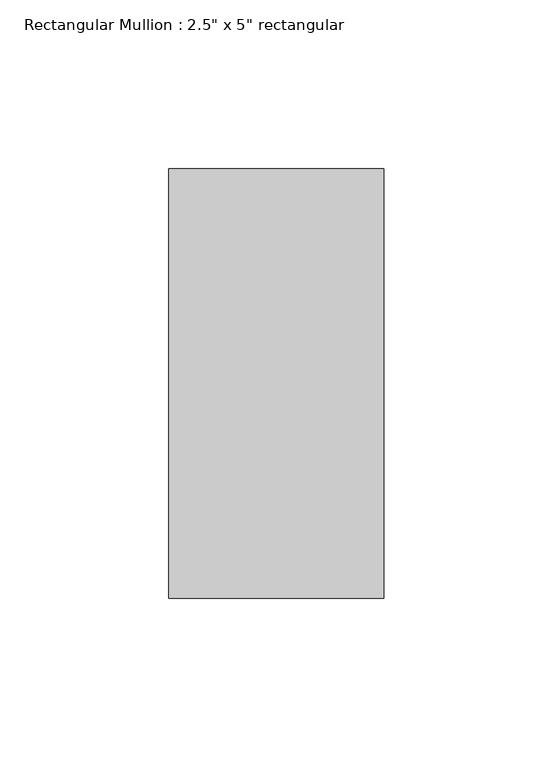
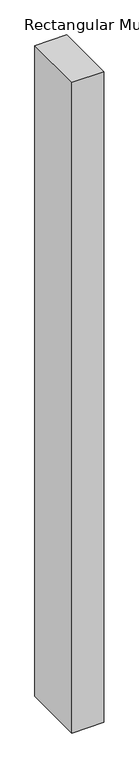
"""IFC4 building model written with IfcOpenShell, lengths in millimetres: member geometry."""

from ifc_helpers import new_model, si_unit, frame, origin, place, context, project, spatial, polyline, outline, extrude, source, transform, mapped, element, save


def member_ef5723a8(model_context):
    return source(origin(), model_context, "Body", "SweptSolid", [
        extrude(outline(polyline([(0.0, 63.5), (0.0, -63.5), (-63.5, -63.5), (-63.5, 63.5), (0.0, 63.5)])), frame((0.0, 0.0, -1365.4610041), z_axis=(0.0, 0.0, 1.0), x_axis=(1.0, 0.0, 0.0)), (0.0, 0.0, 1.0), 1365.4610041),
    ])


if __name__ == "__main__":
    model = new_model("IFC4")
    model_context = context("Model", 3, world=origin())
    ifc_project = project(units=[si_unit("LENGTHUNIT", "METRE", prefix="MILLI")], contexts=[model_context])
    site = spatial("IfcSite", under=ifc_project)
    building = spatial("IfcBuilding", under=site)
    placement = place(None, origin())
    member_shape = member_ef5723a8(model_context)
    element("IfcMember", 1, ObjectType="Rectangular Mullion : 2.5\" x 5\" rectangular", at=placement, inside=building, context=model_context, shape_type="MappedRepresentation", body=[
        mapped(member_shape, transform((0.0, 0.0, 0.0), x_axis=(1.0, 0.0, 0.0), y_axis=(0.0, 1.0, 0.0), z_axis=(0.0, 0.0, 1.0))),
    ])
    save(model, "model.ifc")

# Revit data of these elements
# Type "Rectangular Mullion : 2.5\" x 5\" rectangular"
#   built-in parameter 1007304 = 0.416667 (stored number, unit not read)
#   built-in parameter 1007301 = 0.104167 (stored number, unit not read)
#   built-in parameter 1007300 = 0.104167 (stored number, unit not read)
# Element 1 (IfcMember, "Rectangular Mullion : 2.5\" x 5\" rectangular")
#   Materials on its faces: "Aluminum"
# Materials
#   "Aluminum": class "Metal", colour RGB 247 247 247, transparency 0, Description = "Aluminum 6061", Cost = 0
